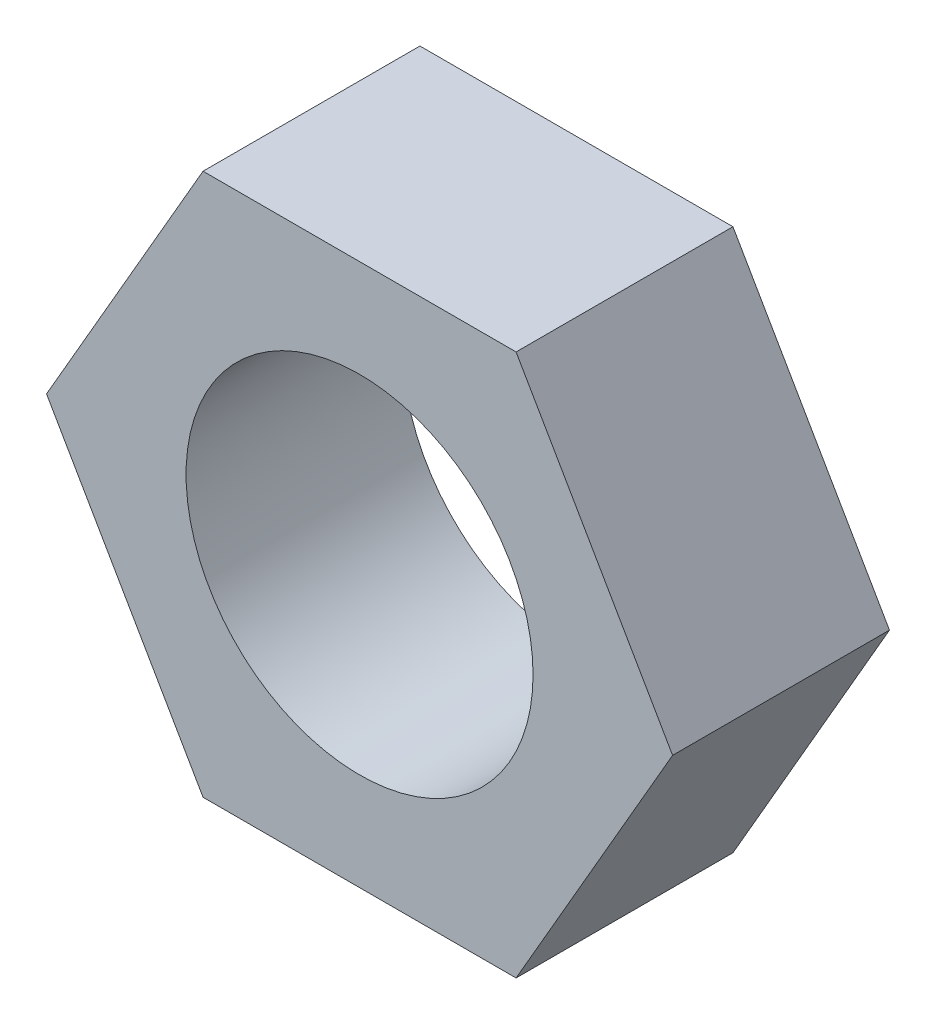
from build123d import *

# Parameters (mm, degrees)
HEX_BODY_25AF_X10_DEPTH = 10
BORE_SKETCH_16_R        = 8
BORE_16_DEPTH           = 10


with BuildPart() as part:
    # Hex Profile Sketch 25AF → Hex Body 25AF x10 (new body)
    with BuildSketch(Plane.XY):
        Polygon((14.43375673, 0), (7.216878365, 12.5), (-7.216878365, 12.5), (-14.43375673, 0), (-7.216878365, -12.5), (7.216878365, -12.5), align=None)
    extrude(amount=HEX_BODY_25AF_X10_DEPTH)

    # Bore Sketch Ø16 → Bore Ø16 (cut)
    with BuildSketch(Plane.XY.offset(10)):
        Circle(BORE_SKETCH_16_R)
    extrude(amount=-BORE_16_DEPTH, mode=Mode.SUBTRACT)


solid = part.part
